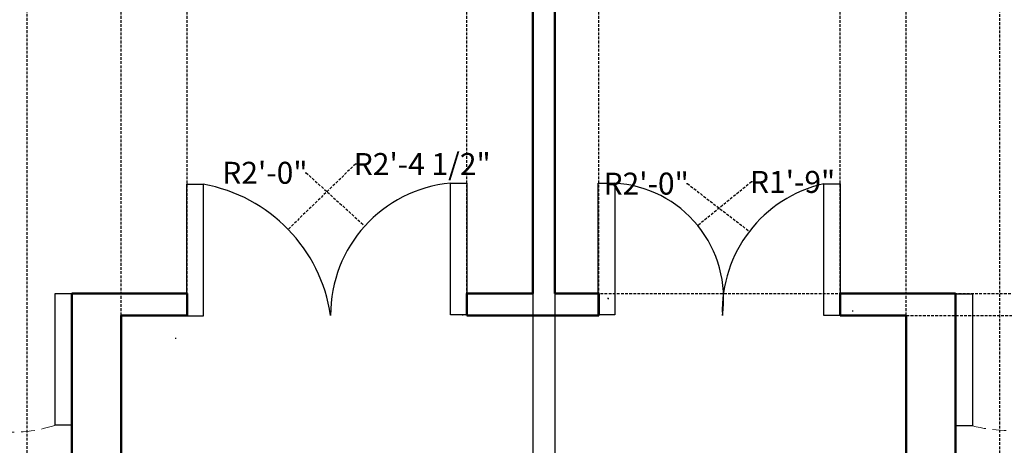
# Model space of a CAD drawing. Units: inches. Extents: x 513 to 1142, y 396 to 927.
# Tile 14 of 31: x 743 to 922, y 614 to 691. Entities that reach past the tile are written whole.
import ezdxf

# ---------------------------------------------------------------- set-up
doc = ezdxf.new("R2010")
doc.units = ezdxf.units.IN
doc.header["$MEASUREMENT"] = 0
doc.linetypes.add('DASHED', pattern=[0.75, 0.5, -0.25])
for name, color, linetype, lineweight in [('A-ANNO-DIMS', 2, 'DASHED', 18), ('A-DOOR', 4, 'Continuous', 25), ('A-DOOR-SWNG', 4, 'DASHED', 13), ('A-WALL', 7, 'Continuous', 50)]:
    doc.layers.add(name, color=color, linetype=linetype, lineweight=lineweight)
doc.styles.get("Standard").update_dxf_attribs({"font": 'arial.ttf'})
doc.dimstyles.get("Standard").update_dxf_attribs({"dimtxt": 4, "dimasz": 0.18, "dimexe": 0.18, "dimexo": 0.0625, "dimgap": 0.09, "dimtad": 0, "dimtih": 1, "dimtoh": 1, "dimdec": 0, "dimrnd": 6, "dimzin": 0, "dimdsep": 46, "dimlunit": 3, "dimtxsty": 'Standard', "dimcen": 0.09, "dimadec": 0, "dimazin": 0, "dimtfac": 1, "dimtdec": 0, "dimtofl": 0, "dimtmove": 0, "dimatfit": 3, "dimfxl": 1, "dimtolj": 1, "dimtzin": 0, "dimarcsym": 0})

# ---------------------------------------------------------------- blocks, each defined once
blk = doc.blocks.new('DOOR-LEAF-24IN')
blk.add_lwpolyline([(3, 24), (3, 0), (0, 0), (0, 24)], close=True)
blk = doc.blocks.new('*D136')
at = {"layer": 'A-ANNO-DIMS', "color": 0, "lineweight": -2, "transparency": 16777216}
for p, q in [((836, 770.1), (836, 401.58)), ((743.8, 768.61), (743.8, 401.58)), ((743.98, 401.76), (784.51, 401.76)), ((835.82, 401.76), (795.29, 401.76))]:
    blk.add_line(p, q, dxfattribs=at)
at = {"layer": 'A-ANNO-DIMS', "color": 0, "transparency": 16777216}
for points in [[(743.98, 401.79), (743.98, 401.73), (743.8, 401.76)], [(835.82, 401.79), (835.82, 401.73), (836, 401.76)]]:
    blk.add_solid(points, dxfattribs=at)
at = {"layer": 'Defpoints', "color": 0, "transparency": 16777216}
for p in [(836, 770.16), (743.8, 768.67), (836, 401.76)]:
    blk.add_point(p, dxfattribs=at)
at = {"layer": 'A-ANNO-DIMS', "color": 0, "transparency": 16777216, "insert": (789.9, 401.76), "char_height": 4, "attachment_point": 5}
blk.add_mtext('\\A1;7\'-8"', dxfattribs=at)
blk = doc.blocks.new('*D137')
at = {"layer": 'A-ANNO-DIMS', "color": 0, "lineweight": -2, "transparency": 16777216}
for p, q in [((840, 770.1), (840, 401.58)), ((921, 770.07), (921, 401.58)), ((840.18, 401.76), (875.08, 401.76)), ((920.82, 401.76), (885.91, 401.76))]:
    blk.add_line(p, q, dxfattribs=at)
at = {"layer": 'A-ANNO-DIMS', "color": 0, "transparency": 16777216}
for points in [[(840.18, 401.79), (840.18, 401.73), (840, 401.76)], [(920.82, 401.79), (920.82, 401.73), (921, 401.76)]]:
    blk.add_solid(points, dxfattribs=at)
at = {"layer": 'Defpoints', "color": 0, "transparency": 16777216}
for p in [(840, 770.16), (921, 770.13), (921, 401.76)]:
    blk.add_point(p, dxfattribs=at)
at = {"layer": 'A-ANNO-DIMS', "color": 0, "transparency": 16777216, "insert": (880.5, 401.76), "char_height": 4, "attachment_point": 5}
blk.add_mtext('\\A1;6\'-9"', dxfattribs=at)
blk = doc.blocks.new('*D149')
at = {"layer": 'A-ANNO-DIMS', "color": 0, "lineweight": -2, "transparency": 16777216}
for p, q in [((840.06, 770.16), (1131.58, 770.16)), ((1131.4, 769.98), (1131.4, 707.79)), ((1131.4, 641.34), (1131.4, 703.53)), ((840.06, 641.16), (1131.58, 641.16))]:
    blk.add_line(p, q, dxfattribs=at)
at = {"layer": 'A-ANNO-DIMS', "color": 0, "transparency": 16777216}
for points in [[(1131.37, 769.98), (1131.43, 769.98), (1131.4, 770.16)], [(1131.37, 641.34), (1131.43, 641.34), (1131.4, 641.16)]]:
    blk.add_solid(points, dxfattribs=at)
at = {"layer": 'Defpoints', "color": 0, "transparency": 16777216}
for p in [(840, 770.16), (1131.4, 770.16), (840, 641.16)]:
    blk.add_point(p, dxfattribs=at)
at = {"layer": 'A-ANNO-DIMS', "color": 0, "transparency": 16777216, "insert": (1131.4, 705.66), "char_height": 4, "attachment_point": 5}
blk.add_mtext('\\A1;10\'-9"', dxfattribs=at)
blk = doc.blocks.new('*D167')
at = {"layer": 'A-ANNO-DIMS', "color": 0, "lineweight": -2, "transparency": 16777216}
for p, q in [((761, 637.22), (761, 920.74)), ((761.18, 920.56), (761.78, 920.56)), ((772.82, 920.56), (772.21, 920.56)), ((773, 637.22), (773, 920.74))]:
    blk.add_line(p, q, dxfattribs=at)
at = {"layer": 'A-ANNO-DIMS', "color": 0, "transparency": 16777216}
for points in [[(761.18, 920.59), (761.18, 920.53), (761, 920.56)], [(772.82, 920.59), (772.82, 920.53), (773, 920.56)]]:
    blk.add_solid(points, dxfattribs=at)
at = {"layer": 'Defpoints', "color": 0, "transparency": 16777216}
for p in [(773, 920.56), (761, 637.16), (773, 637.16)]:
    blk.add_point(p, dxfattribs=at)
at = {"layer": 'A-ANNO-DIMS', "color": 0, "transparency": 16777216, "insert": (767, 920.56), "char_height": 4, "attachment_point": 5}
blk.add_mtext('\\A1;1\'-0"', dxfattribs=at)
blk = doc.blocks.new('*D168')
at = {"layer": 'A-ANNO-DIMS', "color": 0, "lineweight": -2, "transparency": 16777216}
for p, q in [((892, 637.22), (892, 920.74)), ((892.18, 920.56), (892.78, 920.56)), ((903.82, 920.56), (903.21, 920.56)), ((904, 637.22), (904, 920.74))]:
    blk.add_line(p, q, dxfattribs=at)
at = {"layer": 'A-ANNO-DIMS', "color": 0, "transparency": 16777216}
for points in [[(892.18, 920.59), (892.18, 920.53), (892, 920.56)], [(903.82, 920.59), (903.82, 920.53), (904, 920.56)]]:
    blk.add_solid(points, dxfattribs=at)
at = {"layer": 'Defpoints', "color": 0, "transparency": 16777216}
for p in [(904, 920.56), (892, 637.16), (904, 637.16)]:
    blk.add_point(p, dxfattribs=at)
at = {"layer": 'A-ANNO-DIMS', "color": 0, "transparency": 16777216, "insert": (898, 920.56), "char_height": 4, "attachment_point": 5}
blk.add_mtext('\\A1;1\'-0"', dxfattribs=at)
blk = doc.blocks.new('*D169')
at = {"layer": 'A-ANNO-DIMS', "color": 0, "lineweight": -2, "transparency": 16777216}
for p, q in [((836, 774.1), (836, 401.58)), ((840, 774.1), (840, 401.58)), ((836.18, 401.76), (839.82, 401.76)), ((840, 401.76), (840.18, 401.76))]:
    blk.add_line(p, q, dxfattribs=at)
at = {"layer": 'A-ANNO-DIMS', "color": 0, "transparency": 16777216}
for points in [[(836.18, 401.79), (836.18, 401.73), (836, 401.76)], [(839.82, 401.79), (839.82, 401.73), (840, 401.76)]]:
    blk.add_solid(points, dxfattribs=at)
at = {"layer": 'Defpoints', "color": 0, "transparency": 16777216}
for p in [(836, 774.16), (840, 774.16), (840, 401.76)]:
    blk.add_point(p, dxfattribs=at)
at = {"layer": 'A-ANNO-DIMS', "color": 0, "transparency": 16777216, "insert": (845.58, 401.76), "char_height": 4, "attachment_point": 5}
blk.add_mtext('\\A1;0\'-4"', dxfattribs=at)
blk = doc.blocks.new('*D173')
at = {"layer": 'A-ANNO-DIMS', "color": 0, "lineweight": -2, "transparency": 16777216}
for p, q in [((904.06, 637.16), (1131.58, 637.16)), ((1131.4, 636.98), (1131.4, 618.76)), ((1131.4, 596.27), (1131.4, 614.49)), ((904.06, 596.09), (1131.58, 596.09))]:
    blk.add_line(p, q, dxfattribs=at)
at = {"layer": 'A-ANNO-DIMS', "color": 0, "transparency": 16777216}
for points in [[(1131.37, 636.98), (1131.43, 636.98), (1131.4, 637.16)], [(1131.37, 596.27), (1131.43, 596.27), (1131.4, 596.09)]]:
    blk.add_solid(points, dxfattribs=at)
at = {"layer": 'Defpoints', "color": 0, "transparency": 16777216}
for p in [(904, 637.16), (1131.4, 637.16), (904, 596.09)]:
    blk.add_point(p, dxfattribs=at)
at = {"layer": 'A-ANNO-DIMS', "color": 0, "transparency": 16777216, "insert": (1131.4, 616.63), "char_height": 4, "attachment_point": 5}
blk.add_mtext('\\A1;3\'-5"', dxfattribs=at)
blk = doc.blocks.new('*D175')
at = {"layer": 'A-ANNO-DIMS', "color": 0, "lineweight": -2, "transparency": 16777216}
for p, q in [((773, 637.22), (773, 920.74)), ((773.18, 920.56), (793.01, 920.56)), ((823.82, 920.56), (803.98, 920.56)), ((824, 637.22), (824, 920.74))]:
    blk.add_line(p, q, dxfattribs=at)
at = {"layer": 'A-ANNO-DIMS', "color": 0, "transparency": 16777216}
for points in [[(773.18, 920.59), (773.18, 920.53), (773, 920.56)], [(823.82, 920.59), (823.82, 920.53), (824, 920.56)]]:
    blk.add_solid(points, dxfattribs=at)
at = {"layer": 'Defpoints', "color": 0, "transparency": 16777216}
for p in [(824, 920.56), (773, 637.16), (824, 637.16)]:
    blk.add_point(p, dxfattribs=at)
at = {"layer": 'A-ANNO-DIMS', "color": 0, "transparency": 16777216, "insert": (798.5, 920.56), "char_height": 4, "attachment_point": 5}
blk.add_mtext('\\A1;4\'-3"', dxfattribs=at)
blk = doc.blocks.new('*D176')
at = {"layer": 'A-ANNO-DIMS', "color": 0, "lineweight": -2, "transparency": 16777216}
for p, q in [((848, 637.22), (848, 920.74)), ((848.18, 920.56), (864.59, 920.56)), ((891.82, 920.56), (875.4, 920.56)), ((892, 637.22), (892, 920.74))]:
    blk.add_line(p, q, dxfattribs=at)
at = {"layer": 'A-ANNO-DIMS', "color": 0, "transparency": 16777216}
for points in [[(848.18, 920.59), (848.18, 920.53), (848, 920.56)], [(891.82, 920.59), (891.82, 920.53), (892, 920.56)]]:
    blk.add_solid(points, dxfattribs=at)
at = {"layer": 'Defpoints', "color": 0, "transparency": 16777216}
for p in [(892, 920.56), (848, 637.16), (892, 637.16)]:
    blk.add_point(p, dxfattribs=at)
at = {"layer": 'A-ANNO-DIMS', "color": 0, "transparency": 16777216, "insert": (870, 920.56), "char_height": 4, "attachment_point": 5}
blk.add_mtext('\\A1;3\'-8"', dxfattribs=at)
blk = doc.blocks.new('*D177')
at = {"layer": 'A-ANNO-DIMS', "color": 0, "lineweight": -2, "transparency": 16777216}
for p, q in [((803.69, 664.75), (791.54, 652.97)), ((803.87, 664.75), (803.69, 664.75)), ((770.87, 633), (771.05, 633)), ((770.96, 632.91), (770.96, 633.09))]:
    blk.add_line(p, q, dxfattribs=at)
at = {"layer": 'A-ANNO-DIMS', "color": 0, "transparency": 16777216}
blk.add_solid([(791.52, 652.99), (791.56, 652.95), (791.41, 652.85)], dxfattribs=at)
at = {"layer": 'Defpoints', "color": 0, "transparency": 16777216}
for p in [(791.41, 652.85), (770.96, 633)]:
    blk.add_point(p, dxfattribs=at)
at = {"layer": 'A-ANNO-DIMS', "color": 0, "transparency": 16777216, "insert": (815.85, 664.75), "char_height": 4, "attachment_point": 5}
blk.add_mtext('\\A1;R2\'-4 1/2"', dxfattribs=at)
blk = doc.blocks.new('*D184')
at = {"layer": 'A-ANNO-DIMS', "color": 0, "lineweight": -2, "transparency": 16777216}
for p, q in [((794.51, 663.15), (794.69, 663.15)), ((794.69, 663.15), (805.26, 653.57)), ((823.14, 637.28), (823.32, 637.28)), ((823.23, 637.19), (823.23, 637.37))]:
    blk.add_line(p, q, dxfattribs=at)
at = {"layer": 'A-ANNO-DIMS', "color": 0, "transparency": 16777216}
blk.add_solid([(805.28, 653.59), (805.24, 653.55), (805.39, 653.45)], dxfattribs=at)
at = {"layer": 'Defpoints', "color": 0, "transparency": 16777216}
for p in [(805.39, 653.45), (823.23, 637.28)]:
    blk.add_point(p, dxfattribs=at)
at = {"layer": 'A-ANNO-DIMS', "color": 0, "transparency": 16777216, "insert": (787.19, 663.15), "char_height": 4, "attachment_point": 5}
blk.add_mtext('\\A1;R2\'-0"', dxfattribs=at)
blk = doc.blocks.new('*D185')
at = {"layer": 'A-ANNO-DIMS', "color": 0, "lineweight": -2, "transparency": 16777216}
for p, q in [((863.96, 661.18), (864.14, 661.18)), ((864.14, 661.18), (875.29, 652.59)), ((894.18, 637.98), (894.36, 637.98)), ((894.27, 637.89), (894.27, 638.07))]:
    blk.add_line(p, q, dxfattribs=at)
at = {"layer": 'A-ANNO-DIMS', "color": 0, "transparency": 16777216}
blk.add_solid([(875.31, 652.62), (875.28, 652.57), (875.44, 652.48)], dxfattribs=at)
at = {"layer": 'Defpoints', "color": 0, "transparency": 16777216}
for p in [(875.44, 652.48), (894.27, 637.98)]:
    blk.add_point(p, dxfattribs=at)
at = {"layer": 'A-ANNO-DIMS', "color": 0, "transparency": 16777216, "insert": (856.64, 661.18), "char_height": 4, "attachment_point": 5}
blk.add_mtext('\\A1;R2\'-0"', dxfattribs=at)
blk = doc.blocks.new('*D186')
at = {"layer": 'A-ANNO-DIMS', "color": 0, "lineweight": -2, "transparency": 16777216}
for p, q in [((875.82, 661.49), (866.17, 653.64)), ((876, 661.49), (875.82, 661.49)), ((849.72, 640.17), (849.72, 640.35)), ((849.63, 640.26), (849.81, 640.26))]:
    blk.add_line(p, q, dxfattribs=at)
at = {"layer": 'A-ANNO-DIMS', "color": 0, "transparency": 16777216}
blk.add_solid([(866.15, 653.66), (866.19, 653.62), (866.03, 653.52)], dxfattribs=at)
at = {"layer": 'Defpoints', "color": 0, "transparency": 16777216}
for p in [(866.03, 653.52), (849.72, 640.26)]:
    blk.add_point(p, dxfattribs=at)
at = {"layer": 'A-ANNO-DIMS', "color": 0, "transparency": 16777216, "insert": (883.32, 661.49), "char_height": 4, "attachment_point": 5}
blk.add_mtext('\\A1;R1\'-9"', dxfattribs=at)

msp = doc.modelspace()

# ---------------------------------------------------------------- linework, layer by layer
at = {"layer": 'A-DOOR'}
for centre, radius, start, end in [((770.96, 633), 28.5, 8.3914, 79.874), ((823.23, 637.28), 24.08, 95.3306, 180.2805), ((849.72, 640.26), 21.03, 351.5244, 86.72), ((894.27, 637.98), 23.77, 102.8181, 181.9864)]:
    msp.add_arc(centre, radius, start, end, dxfattribs=at)
at = {"layer": 'A-DOOR-SWNG', "ltscale": 5}
for centre, radius, start, end in [((741.15, 641.06), 25.16, 179.7799, 288.1654), ((922.84, 642.37), 26.18, 254.9757, 357.339)]:
    msp.add_arc(centre, radius, start, end, dxfattribs=at)
at = {"layer": 'A-WALL'}
for p, q in [((836, 770.16), (836, 641.16)), ((840, 770.16), (840, 641.16)), ((752, 641.16), (752, 497.16)), ((752, 641.16), (773, 641.16)), ((773, 641.16), (773, 637.16)), ((824, 641.16), (824, 637.16)), ((824, 641.16), (836, 641.16)), ((840, 641.16), (848, 641.16)), ((848, 641.16), (848, 637.16)), ((892, 637.16), (892, 641.16)), ((892, 641.16), (913, 641.16)), ((913, 497.16), (913, 641.16)), ((761, 637.16), (761, 473.16)), ((761, 637.16), (773, 637.16)), ((824, 637.16), (836, 637.16)), ((836, 637.16), (848, 637.16)), ((892, 637.16), (904, 637.16)), ((904, 473.16), (904, 637.16))]:
    msp.add_line(p, q, dxfattribs=at)

# ---------------------------------------------------------------- block references
at = {"layer": 'A-DOOR'}
for p in [(772.97, 637.06), (820.99, 637.25), (847.92, 637.25), (889, 637.16), (913.06, 617.09)]:
    msp.add_blockref('DOOR-LEAF-24IN', p, dxfattribs=at)
at = {"layer": 'A-DOOR', "rotation": 180}
msp.add_blockref('DOOR-LEAF-24IN', (752, 641.16), dxfattribs=at)

# ---------------------------------------------------------------- dimensions: what is measured, and where the dimension line sits
at = {"layer": 'A-ANNO-DIMS'}
for base, p1, p2, picture, middle in [((773, 920.56), (761, 637.16), (773, 637.16), '*D167', (767, 920.56)), ((824, 920.56), (773, 637.16), (824, 637.16), '*D175', (798.5, 920.56)), ((892, 920.56), (848, 637.16), (892, 637.16), '*D176', (870, 920.56)), ((904, 920.56), (892, 637.16), (904, 637.16), '*D168', (898, 920.56)), ((840, 401.76), (836, 774.16), (840, 774.16), '*D169', (845.58, 401.76)), ((836, 401.76), (743.8, 768.67), (836, 770.16), '*D136', (789.9, 401.76)), ((921, 401.76), (840, 770.16), (921, 770.13), '*D137', (880.5, 401.76))]:
    dim = msp.add_linear_dim(base=base, p1=p1, p2=p2, dimstyle='Standard', override={"dimdec": 1, "dimlfac": 1, "dimrnd": 0, "dimzin": 1, "dimdsep": 46, "dimlunit": 4, "dimfrac": 2}, dxfattribs=at)
    dim.commit()
    dim.dimension.update_dxf_attribs({"geometry": picture, "text_midpoint": middle})
for base, p1, p2, picture, middle in [((1131.4, 770.16), (840, 641.16), (840, 770.16), '*D149', (1131.4, 705.66)), ((1131.4, 637.16), (904, 596.09), (904, 637.16), '*D173', (1131.4, 616.63))]:
    dim = msp.add_linear_dim(base=base, p1=p1, p2=p2, angle=90, dimstyle='Standard', override={"dimdec": 1, "dimlfac": 1, "dimrnd": 0, "dimzin": 1, "dimdsep": 46, "dimlunit": 4, "dimfrac": 2}, dxfattribs=at)
    dim.commit()
    dim.dimension.update_dxf_attribs({"geometry": picture, "text_midpoint": middle})
for center, mpoint, picture, middle in [((770.96, 633), (791.41, 652.85), '*D177', (815.85, 664.75)), ((823.23, 637.28), (805.39, 653.45), '*D184', (787.19, 663.15)), ((894.27, 637.98), (875.44, 652.48), '*D185', (856.64, 661.18)), ((849.72, 640.26), (866.03, 653.52), '*D186', (883.32, 661.49))]:
    dim = msp.add_radius_dim(center=center, mpoint=mpoint, dimstyle='Standard', override={"dimdec": 1, "dimlfac": 1, "dimrnd": 0, "dimzin": 1, "dimdsep": 46, "dimlunit": 4, "dimfrac": 2}, dxfattribs=at)
    dim.commit()
    dim.dimension.update_dxf_attribs({"geometry": picture, "text_midpoint": middle, "dimtype": 164})

doc.saveas('drawing.dxf')
